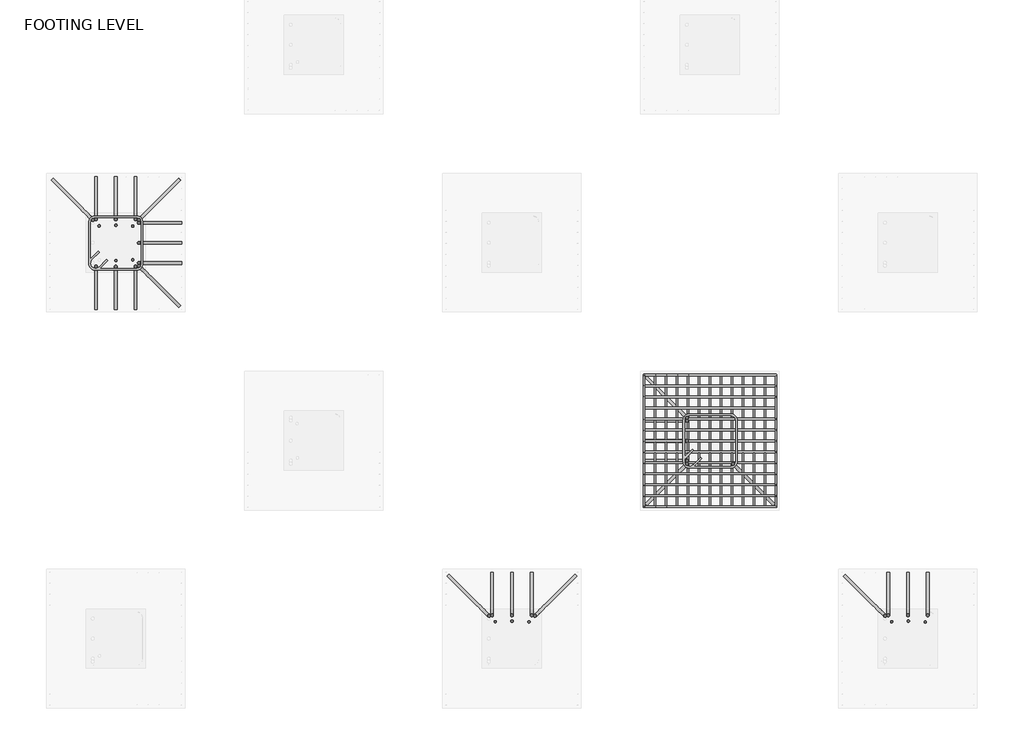
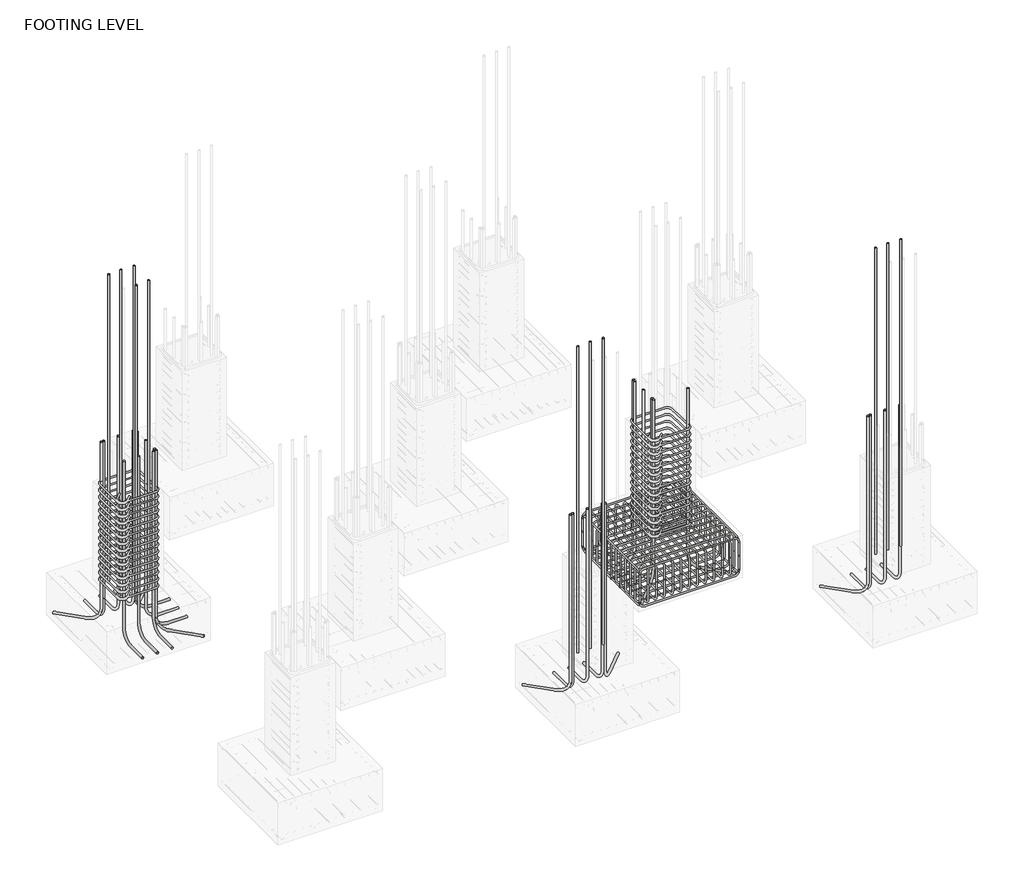
# One storey, part 5 of 10: 33 reinforcing bars.
"""IFC4 building model written with IfcOpenShell, lengths in millimetres."""

from ifc_helpers import new_model, si_unit, point, frame, origin, place, context, project, spatial, polyline, circle_curve, trimmed, segment, composite_curve, source, transform, mapped, element, save
from ifc_brep_helpers import swept_disk

model = new_model("IFC4")

# Units and contexts
model_context = context("Model", 3, world=origin())
ifc_project = project(units=[si_unit("LENGTHUNIT", "METRE", prefix="MILLI")], contexts=[model_context])

# Site, building, storey
site = spatial("IfcSite", under=ifc_project)
building = spatial("IfcBuilding", under=site)
storey = spatial("IfcBuildingStorey", under=building, Name="FOOTING LEVEL", Elevation=-2133.6)

# Reinforcing bars
placement = place(None, origin())
reinforcing_bar_shape = source(origin(), model_context, "Body", "SolidModel", [
    swept_disk(composite_curve([segment(polyline([(-2682.9269037, 3804.4829396, -2583.0), (-2682.9269037, 3804.4829396, -2905.1)]), True, "CONTINUOUS"), segment(trimmed(circle_curve(frame((-2773.1269037, 3804.4829396, -2905.1), z_axis=(0.0, 1.0, 0.0), x_axis=(90.20000000000027, 0.0, 0.0)), 90.2), [point((-2682.9269037, 3804.4829396, -2905.1))], [point((-2773.1269037, 3804.4829396, -2995.3))], True, "CARTESIAN"), True, "CONTINUOUS"), segment(polyline([(-2773.1269037, 3804.4829396, -2995.3), (-4620.9269037, 3804.4829396, -2995.3)]), True, "CONTINUOUS"), segment(trimmed(circle_curve(frame((-4620.9269037, 3804.4829396, -2905.1), z_axis=(0.0, 1.0, 0.0), x_axis=(0.0, 0.0, -90.20000000000027)), 90.2), [point((-4620.9269037, 3804.4829396, -2995.3))], [point((-4711.1269037, 3804.4829396, -2905.1))], True, "CARTESIAN"), True, "CONTINUOUS"), segment(polyline([(-4711.1269037, 3804.4829396, -2905.1), (-4711.1269037, 3804.4829396, -2583.0)]), True, "CONTINUOUS")], self_intersect=False), 12.7),
])
element("IfcReinforcingBar", 1, at=placement, inside=storey, context=model_context, shape_type="MappedRepresentation", body=[
    mapped(reinforcing_bar_shape, transform((0.0, 0.0, 0.0), x_axis=(1.0, 0.0, 0.0), y_axis=(0.0, 1.0, 0.0), z_axis=(0.0, 0.0, 1.0))),
    mapped(reinforcing_bar_shape, transform((0.0, -169.0166667, 0.0), x_axis=(1.0, 0.0, 0.0), y_axis=(0.0, 1.0, 0.0), z_axis=(0.0, 0.0, 1.0))),
    mapped(reinforcing_bar_shape, transform((0.0, -338.0333333, 0.0), x_axis=(1.0, 0.0, 0.0), y_axis=(0.0, 1.0, 0.0), z_axis=(0.0, 0.0, 1.0))),
    mapped(reinforcing_bar_shape, transform((0.0, -507.05, 0.0), x_axis=(1.0, 0.0, 0.0), y_axis=(0.0, 1.0, 0.0), z_axis=(0.0, 0.0, 1.0))),
    mapped(reinforcing_bar_shape, transform((0.0, -676.0666667, 0.0), x_axis=(1.0, 0.0, 0.0), y_axis=(0.0, 1.0, 0.0), z_axis=(0.0, 0.0, 1.0))),
    mapped(reinforcing_bar_shape, transform((0.0, -845.0833333, 0.0), x_axis=(1.0, 0.0, 0.0), y_axis=(0.0, 1.0, 0.0), z_axis=(0.0, 0.0, 1.0))),
    mapped(reinforcing_bar_shape, transform((0.0, -1014.1, 0.0), x_axis=(1.0, 0.0, 0.0), y_axis=(0.0, 1.0, 0.0), z_axis=(0.0, 0.0, 1.0))),
    mapped(reinforcing_bar_shape, transform((0.0, -1183.1166667, 0.0), x_axis=(1.0, 0.0, 0.0), y_axis=(0.0, 1.0, 0.0), z_axis=(0.0, 0.0, 1.0))),
    mapped(reinforcing_bar_shape, transform((0.0, -1352.1333333, 0.0), x_axis=(1.0, 0.0, 0.0), y_axis=(0.0, 1.0, 0.0), z_axis=(0.0, 0.0, 1.0))),
    mapped(reinforcing_bar_shape, transform((0.0, -1521.15, 0.0), x_axis=(1.0, 0.0, 0.0), y_axis=(0.0, 1.0, 0.0), z_axis=(0.0, 0.0, 1.0))),
    mapped(reinforcing_bar_shape, transform((0.0, -1690.1666667, 0.0), x_axis=(1.0, 0.0, 0.0), y_axis=(0.0, 1.0, 0.0), z_axis=(0.0, 0.0, 1.0))),
    mapped(reinforcing_bar_shape, transform((0.0, -1859.1833333, 0.0), x_axis=(1.0, 0.0, 0.0), y_axis=(0.0, 1.0, 0.0), z_axis=(0.0, 0.0, 1.0))),
    mapped(reinforcing_bar_shape, transform((0.0, -2028.2, 0.0), x_axis=(1.0, 0.0, 0.0), y_axis=(0.0, 1.0, 0.0), z_axis=(0.0, 0.0, 1.0))),
])
reinforcing_bar_2_shape = source(origin(), model_context, "Body", "SolidModel", [
    swept_disk(composite_curve([segment(polyline([(-4711.1269037, 3804.4829396, -2598.6), (-4711.1269037, 3804.4829396, -2276.5)]), True, "CONTINUOUS"), segment(trimmed(circle_curve(frame((-4620.9269037, 3804.4829396, -2276.5), z_axis=(0.0, 1.0, 0.0), x_axis=(-90.19999999999982, 0.0, 0.0)), 90.2), [point((-4711.1269037, 3804.4829396, -2276.5))], [point((-4620.9269037, 3804.4829396, -2186.3))], True, "CARTESIAN"), True, "CONTINUOUS"), segment(polyline([(-4620.9269037, 3804.4829396, -2186.3), (-2773.1269037, 3804.4829396, -2186.3)]), True, "CONTINUOUS"), segment(trimmed(circle_curve(frame((-2773.1269037, 3804.4829396, -2276.5), z_axis=(0.0, 1.0, 0.0), x_axis=(0.0, 0.0, 90.19999999999982)), 90.2), [point((-2773.1269037, 3804.4829396, -2186.3))], [point((-2682.9269037, 3804.4829396, -2276.5))], True, "CARTESIAN"), True, "CONTINUOUS"), segment(polyline([(-2682.9269037, 3804.4829396, -2276.5), (-2682.9269037, 3804.4829396, -2598.6)]), True, "CONTINUOUS")], self_intersect=False), 12.7),
])
element("IfcReinforcingBar", 2, at=placement, inside=storey, context=model_context, shape_type="MappedRepresentation", body=[
    mapped(reinforcing_bar_2_shape, transform((0.0, 0.0, 0.0), x_axis=(1.0, 0.0, 0.0), y_axis=(0.0, 1.0, 0.0), z_axis=(0.0, 0.0, 1.0))),
    mapped(reinforcing_bar_2_shape, transform((0.0, -169.0166667, 0.0), x_axis=(1.0, 0.0, 0.0), y_axis=(0.0, 1.0, 0.0), z_axis=(0.0, 0.0, 1.0))),
    mapped(reinforcing_bar_2_shape, transform((0.0, -338.0333333, 0.0), x_axis=(1.0, 0.0, 0.0), y_axis=(0.0, 1.0, 0.0), z_axis=(0.0, 0.0, 1.0))),
    mapped(reinforcing_bar_2_shape, transform((0.0, -507.05, 0.0), x_axis=(1.0, 0.0, 0.0), y_axis=(0.0, 1.0, 0.0), z_axis=(0.0, 0.0, 1.0))),
    mapped(reinforcing_bar_2_shape, transform((0.0, -676.0666667, 0.0), x_axis=(1.0, 0.0, 0.0), y_axis=(0.0, 1.0, 0.0), z_axis=(0.0, 0.0, 1.0))),
    mapped(reinforcing_bar_2_shape, transform((0.0, -845.0833333, 0.0), x_axis=(1.0, 0.0, 0.0), y_axis=(0.0, 1.0, 0.0), z_axis=(0.0, 0.0, 1.0))),
    mapped(reinforcing_bar_2_shape, transform((0.0, -1014.1, 0.0), x_axis=(1.0, 0.0, 0.0), y_axis=(0.0, 1.0, 0.0), z_axis=(0.0, 0.0, 1.0))),
    mapped(reinforcing_bar_2_shape, transform((0.0, -1183.1166667, 0.0), x_axis=(1.0, 0.0, 0.0), y_axis=(0.0, 1.0, 0.0), z_axis=(0.0, 0.0, 1.0))),
    mapped(reinforcing_bar_2_shape, transform((0.0, -1352.1333333, 0.0), x_axis=(1.0, 0.0, 0.0), y_axis=(0.0, 1.0, 0.0), z_axis=(0.0, 0.0, 1.0))),
    mapped(reinforcing_bar_2_shape, transform((0.0, -1521.15, 0.0), x_axis=(1.0, 0.0, 0.0), y_axis=(0.0, 1.0, 0.0), z_axis=(0.0, 0.0, 1.0))),
    mapped(reinforcing_bar_2_shape, transform((0.0, -1690.1666667, 0.0), x_axis=(1.0, 0.0, 0.0), y_axis=(0.0, 1.0, 0.0), z_axis=(0.0, 0.0, 1.0))),
    mapped(reinforcing_bar_2_shape, transform((0.0, -1859.1833333, 0.0), x_axis=(1.0, 0.0, 0.0), y_axis=(0.0, 1.0, 0.0), z_axis=(0.0, 0.0, 1.0))),
    mapped(reinforcing_bar_2_shape, transform((0.0, -2028.2, 0.0), x_axis=(1.0, 0.0, 0.0), y_axis=(0.0, 1.0, 0.0), z_axis=(0.0, 0.0, 1.0))),
])
reinforcing_bar_3_shape = source(origin(), model_context, "Body", "SolidModel", [
    swept_disk(composite_curve([segment(polyline([(-2682.9269037, 1776.2829396, -2559.4978077), (-2682.9269037, 1776.2829396, -2881.5978077)]), True, "CONTINUOUS"), segment(trimmed(circle_curve(frame((-2682.9269037, 1866.4829396, -2881.5978077), z_axis=(1.0, 0.0, 0.0), x_axis=(0.0, -90.20000000000005, 0.0)), 90.2), [point((-2682.9269037, 1776.2829396, -2881.5978077))], [point((-2682.9269037, 1866.4829396, -2971.7978077))], True, "CARTESIAN"), True, "CONTINUOUS"), segment(polyline([(-2682.9269037, 1866.4829396, -2971.7978077), (-2682.9269037, 3714.2829396, -2971.7978077)]), True, "CONTINUOUS"), segment(trimmed(circle_curve(frame((-2682.9269037, 3714.2829396, -2881.5978077), z_axis=(1.0, 0.0, 0.0), x_axis=(0.0, 0.0, -90.19999999999982)), 90.2), [point((-2682.9269037, 3714.2829396, -2971.7978077))], [point((-2682.9269037, 3804.4829396, -2881.5978077))], True, "CARTESIAN"), True, "CONTINUOUS"), segment(polyline([(-2682.9269037, 3804.4829396, -2881.5978077), (-2682.9269037, 3804.4829396, -2559.4978077)]), True, "CONTINUOUS")], self_intersect=False), 12.7),
])
element("IfcReinforcingBar", 3, at=placement, inside=storey, context=model_context, shape_type="MappedRepresentation", body=[
    mapped(reinforcing_bar_3_shape, transform((0.0, 0.0, 0.0), x_axis=(1.0, 0.0, 0.0), y_axis=(0.0, 1.0, 0.0), z_axis=(0.0, 0.0, 1.0))),
    mapped(reinforcing_bar_3_shape, transform((-169.0166667, 0.0, 0.0), x_axis=(1.0, 0.0, 0.0), y_axis=(0.0, 1.0, 0.0), z_axis=(0.0, 0.0, 1.0))),
    mapped(reinforcing_bar_3_shape, transform((-338.0333333, 0.0, 0.0), x_axis=(1.0, 0.0, 0.0), y_axis=(0.0, 1.0, 0.0), z_axis=(0.0, 0.0, 1.0))),
    mapped(reinforcing_bar_3_shape, transform((-507.05, 0.0, 0.0), x_axis=(1.0, 0.0, 0.0), y_axis=(0.0, 1.0, 0.0), z_axis=(0.0, 0.0, 1.0))),
    mapped(reinforcing_bar_3_shape, transform((-676.0666667, 0.0, 0.0), x_axis=(1.0, 0.0, 0.0), y_axis=(0.0, 1.0, 0.0), z_axis=(0.0, 0.0, 1.0))),
    mapped(reinforcing_bar_3_shape, transform((-845.0833333, 0.0, 0.0), x_axis=(1.0, 0.0, 0.0), y_axis=(0.0, 1.0, 0.0), z_axis=(0.0, 0.0, 1.0))),
    mapped(reinforcing_bar_3_shape, transform((-1014.1, 0.0, 0.0), x_axis=(1.0, 0.0, 0.0), y_axis=(0.0, 1.0, 0.0), z_axis=(0.0, 0.0, 1.0))),
    mapped(reinforcing_bar_3_shape, transform((-1183.1166667, 0.0, 0.0), x_axis=(1.0, 0.0, 0.0), y_axis=(0.0, 1.0, 0.0), z_axis=(0.0, 0.0, 1.0))),
    mapped(reinforcing_bar_3_shape, transform((-1352.1333333, 0.0, 0.0), x_axis=(1.0, 0.0, 0.0), y_axis=(0.0, 1.0, 0.0), z_axis=(0.0, 0.0, 1.0))),
    mapped(reinforcing_bar_3_shape, transform((-1521.15, 0.0, 0.0), x_axis=(1.0, 0.0, 0.0), y_axis=(0.0, 1.0, 0.0), z_axis=(0.0, 0.0, 1.0))),
    mapped(reinforcing_bar_3_shape, transform((-1690.1666667, 0.0, 0.0), x_axis=(1.0, 0.0, 0.0), y_axis=(0.0, 1.0, 0.0), z_axis=(0.0, 0.0, 1.0))),
    mapped(reinforcing_bar_3_shape, transform((-1859.1833333, 0.0, 0.0), x_axis=(1.0, 0.0, 0.0), y_axis=(0.0, 1.0, 0.0), z_axis=(0.0, 0.0, 1.0))),
    mapped(reinforcing_bar_3_shape, transform((-2028.2, 0.0, 0.0), x_axis=(1.0, 0.0, 0.0), y_axis=(0.0, 1.0, 0.0), z_axis=(0.0, 0.0, 1.0))),
])
reinforcing_bar_4_shape = source(origin(), model_context, "Body", "SolidModel", [
    swept_disk(composite_curve([segment(polyline([(-4711.1269037, 1776.2829396, -2622.9919875), (-4711.1269037, 1776.2829396, -2300.8919875)]), True, "CONTINUOUS"), segment(trimmed(circle_curve(frame((-4711.1269037, 1866.4829396, -2300.8919875), z_axis=(-1.0, 0.0, 0.0), x_axis=(0.0, -90.20000000000005, 0.0)), 90.2), [point((-4711.1269037, 1776.2829396, -2300.8919875))], [point((-4711.1269037, 1866.4829396, -2210.6919875))], True, "CARTESIAN"), True, "CONTINUOUS"), segment(polyline([(-4711.1269037, 1866.4829396, -2210.6919875), (-4711.1269037, 3714.2829396, -2210.6919875)]), True, "CONTINUOUS"), segment(trimmed(circle_curve(frame((-4711.1269037, 3714.2829396, -2300.8919875), z_axis=(-1.0, 0.0, 0.0), x_axis=(0.0, 0.0, 90.20000000000027)), 90.2), [point((-4711.1269037, 3714.2829396, -2210.6919875))], [point((-4711.1269037, 3804.4829396, -2300.8919875))], True, "CARTESIAN"), True, "CONTINUOUS"), segment(polyline([(-4711.1269037, 3804.4829396, -2300.8919875), (-4711.1269037, 3804.4829396, -2622.9919875)]), True, "CONTINUOUS")], self_intersect=False), 12.7),
])
element("IfcReinforcingBar", 4, at=placement, inside=storey, context=model_context, shape_type="MappedRepresentation", body=[
    mapped(reinforcing_bar_4_shape, transform((0.0, 0.0, 0.0), x_axis=(1.0, 0.0, 0.0), y_axis=(0.0, 1.0, 0.0), z_axis=(0.0, 0.0, 1.0))),
    mapped(reinforcing_bar_4_shape, transform((169.0166667, 0.0, 0.0), x_axis=(1.0, 0.0, 0.0), y_axis=(0.0, 1.0, 0.0), z_axis=(0.0, 0.0, 1.0))),
    mapped(reinforcing_bar_4_shape, transform((338.0333333, 0.0, 0.0), x_axis=(1.0, 0.0, 0.0), y_axis=(0.0, 1.0, 0.0), z_axis=(0.0, 0.0, 1.0))),
    mapped(reinforcing_bar_4_shape, transform((507.05, 0.0, 0.0), x_axis=(1.0, 0.0, 0.0), y_axis=(0.0, 1.0, 0.0), z_axis=(0.0, 0.0, 1.0))),
    mapped(reinforcing_bar_4_shape, transform((676.0666667, 0.0, 0.0), x_axis=(1.0, 0.0, 0.0), y_axis=(0.0, 1.0, 0.0), z_axis=(0.0, 0.0, 1.0))),
    mapped(reinforcing_bar_4_shape, transform((845.0833333, 0.0, 0.0), x_axis=(1.0, 0.0, 0.0), y_axis=(0.0, 1.0, 0.0), z_axis=(0.0, 0.0, 1.0))),
    mapped(reinforcing_bar_4_shape, transform((1014.1, 0.0, 0.0), x_axis=(1.0, 0.0, 0.0), y_axis=(0.0, 1.0, 0.0), z_axis=(0.0, 0.0, 1.0))),
    mapped(reinforcing_bar_4_shape, transform((1183.1166667, 0.0, 0.0), x_axis=(1.0, 0.0, 0.0), y_axis=(0.0, 1.0, 0.0), z_axis=(0.0, 0.0, 1.0))),
    mapped(reinforcing_bar_4_shape, transform((1352.1333333, 0.0, 0.0), x_axis=(1.0, 0.0, 0.0), y_axis=(0.0, 1.0, 0.0), z_axis=(0.0, 0.0, 1.0))),
    mapped(reinforcing_bar_4_shape, transform((1521.15, 0.0, 0.0), x_axis=(1.0, 0.0, 0.0), y_axis=(0.0, 1.0, 0.0), z_axis=(0.0, 0.0, 1.0))),
    mapped(reinforcing_bar_4_shape, transform((1690.1666667, 0.0, 0.0), x_axis=(1.0, 0.0, 0.0), y_axis=(0.0, 1.0, 0.0), z_axis=(0.0, 0.0, 1.0))),
    mapped(reinforcing_bar_4_shape, transform((1859.1833333, 0.0, 0.0), x_axis=(1.0, 0.0, 0.0), y_axis=(0.0, 1.0, 0.0), z_axis=(0.0, 0.0, 1.0))),
    mapped(reinforcing_bar_4_shape, transform((2028.2, 0.0, 0.0), x_axis=(1.0, 0.0, 0.0), y_axis=(0.0, 1.0, 0.0), z_axis=(0.0, 0.0, 1.0))),
])
reinforcing_bar_5_shape = source(origin(), model_context, "Body", "SolidModel", [
    swept_disk(composite_curve([segment(polyline([(-12978.1462687, 5573.7015113, 0.0), (-13091.545872, 5460.3019079, 0.0)]), True, "CONTINUOUS"), segment(trimmed(circle_curve(frame((-13155.3269037, 5524.0829396, 0.0), z_axis=(0.0, 0.0, -1.0), x_axis=(63.78103169999849, -63.78103170000031, 0.0)), 90.2), [point((-13091.545872, 5460.3019079, 0.0))], [point((-13245.5269037, 5524.0829396, 0.0))], True, "CARTESIAN"), True, "CONTINUOUS"), segment(polyline([(-13245.5269037, 5524.0829396, 0.0), (-13245.5269037, 6152.6829396, 0.0)]), True, "CONTINUOUS"), segment(trimmed(circle_curve(frame((-13155.3269037, 6152.6829396, 0.0), z_axis=(0.0, 0.0, -1.0), x_axis=(-90.20000000000073, 0.0, 0.0)), 90.2), [point((-13245.5269037, 6152.6829396, 0.0))], [point((-13155.3269037, 6242.8829396, 0.0))], True, "CARTESIAN"), True, "CONTINUOUS"), segment(polyline([(-13155.3269037, 6242.8829396, 0.0), (-12526.7269037, 6242.8829396, 0.0)]), True, "CONTINUOUS"), segment(trimmed(circle_curve(frame((-12526.7269037, 6152.7273645, 2.8305953), z_axis=(0.0, -0.03138132276777647, -0.9995074850051623), x_axis=(0.0, 90.15557510000053, -2.8305953)), 90.2), [point((-12526.7269037, 6242.8829396, 0.0))], [point((-12436.5269037, 6152.7273645, 2.8305953))], True, "CARTESIAN"), True, "CONTINUOUS"), segment(polyline([(-12436.5269037, 6152.7273645, 2.8305953), (-12436.5269037, 5524.0385147, 22.5694047)]), True, "CONTINUOUS"), segment(trimmed(circle_curve(frame((-12526.7269037, 5524.0385147, 22.5694047), z_axis=(0.0, -0.03138132276777647, -0.9995074850051623), x_axis=(90.20000000000073, 0.0, 0.0)), 90.2), [point((-12436.5269037, 5524.0385147, 22.5694047))], [point((-12526.7269037, 5433.8829396, 25.4))], True, "CARTESIAN"), True, "CONTINUOUS"), segment(polyline([(-12526.7269037, 5433.8829396, 25.4), (-13155.3269037, 5433.8829396, 25.4)]), True, "CONTINUOUS"), segment(trimmed(circle_curve(frame((-13155.3269037, 5524.0829396, 25.4), z_axis=(0.0, 0.0, -1.0), x_axis=(0.0, -90.19999999999982, 0.0)), 90.2), [point((-13155.3269037, 5433.8829396, 25.4))], [point((-13219.1079353, 5587.8639713, 25.4))], True, "CARTESIAN"), True, "CONTINUOUS"), segment(polyline([(-13219.1079353, 5587.8639713, 25.4), (-13105.708332, 5701.2635746, 25.4)]), True, "CONTINUOUS")], self_intersect=False), 12.7),
])
element("IfcReinforcingBar", 5, at=placement, inside=storey, context=model_context, shape_type="MappedRepresentation", body=[
    mapped(reinforcing_bar_5_shape, transform((0.0, 0.0, 0.0), x_axis=(1.0, 0.0, 0.0), y_axis=(0.0, 1.0, 0.0), z_axis=(0.0, 0.0, 1.0))),
    mapped(reinforcing_bar_5_shape, transform((0.0, 0.0, -148.6357143), x_axis=(1.0, 0.0, 0.0), y_axis=(0.0, 1.0, 0.0), z_axis=(0.0, 0.0, 1.0))),
    mapped(reinforcing_bar_5_shape, transform((0.0, 0.0, -297.2714286), x_axis=(1.0, 0.0, 0.0), y_axis=(0.0, 1.0, 0.0), z_axis=(0.0, 0.0, 1.0))),
    mapped(reinforcing_bar_5_shape, transform((0.0, 0.0, -445.9071429), x_axis=(1.0, 0.0, 0.0), y_axis=(0.0, 1.0, 0.0), z_axis=(0.0, 0.0, 1.0))),
    mapped(reinforcing_bar_5_shape, transform((0.0, 0.0, -594.5428571), x_axis=(1.0, 0.0, 0.0), y_axis=(0.0, 1.0, 0.0), z_axis=(0.0, 0.0, 1.0))),
    mapped(reinforcing_bar_5_shape, transform((0.0, 0.0, -743.1785714), x_axis=(1.0, 0.0, 0.0), y_axis=(0.0, 1.0, 0.0), z_axis=(0.0, 0.0, 1.0))),
    mapped(reinforcing_bar_5_shape, transform((0.0, 0.0, -891.8142857), x_axis=(1.0, 0.0, 0.0), y_axis=(0.0, 1.0, 0.0), z_axis=(0.0, 0.0, 1.0))),
    mapped(reinforcing_bar_5_shape, transform((0.0, 0.0, -1040.45), x_axis=(1.0, 0.0, 0.0), y_axis=(0.0, 1.0, 0.0), z_axis=(0.0, 0.0, 1.0))),
    mapped(reinforcing_bar_5_shape, transform((0.0, 0.0, -1189.0857143), x_axis=(1.0, 0.0, 0.0), y_axis=(0.0, 1.0, 0.0), z_axis=(0.0, 0.0, 1.0))),
    mapped(reinforcing_bar_5_shape, transform((0.0, 0.0, -1337.7214286), x_axis=(1.0, 0.0, 0.0), y_axis=(0.0, 1.0, 0.0), z_axis=(0.0, 0.0, 1.0))),
    mapped(reinforcing_bar_5_shape, transform((0.0, 0.0, -1486.3571429), x_axis=(1.0, 0.0, 0.0), y_axis=(0.0, 1.0, 0.0), z_axis=(0.0, 0.0, 1.0))),
    mapped(reinforcing_bar_5_shape, transform((0.0, 0.0, -1634.9928571), x_axis=(1.0, 0.0, 0.0), y_axis=(0.0, 1.0, 0.0), z_axis=(0.0, 0.0, 1.0))),
    mapped(reinforcing_bar_5_shape, transform((0.0, 0.0, -1783.6285714), x_axis=(1.0, 0.0, 0.0), y_axis=(0.0, 1.0, 0.0), z_axis=(0.0, 0.0, 1.0))),
    mapped(reinforcing_bar_5_shape, transform((0.0, 0.0, -1932.2642857), x_axis=(1.0, 0.0, 0.0), y_axis=(0.0, 1.0, 0.0), z_axis=(0.0, 0.0, 1.0))),
    mapped(reinforcing_bar_5_shape, transform((0.0, 0.0, -2080.9), x_axis=(1.0, 0.0, 0.0), y_axis=(0.0, 1.0, 0.0), z_axis=(0.0, 0.0, 1.0))),
])
reinforcing_bar_6_shape = source(origin(), model_context, "Body", "SolidModel", [
    swept_disk(composite_curve([segment(polyline([(-3834.1462687, 2525.7015113, 0.0), (-3947.545872, 2412.3019079, 0.0)]), True, "CONTINUOUS"), segment(trimmed(circle_curve(frame((-4011.3269037, 2476.0829396, 0.0), z_axis=(0.0, 0.0, -1.0), x_axis=(63.78103169999986, -63.78103169999986, 0.0)), 90.2), [point((-3947.545872, 2412.3019079, 0.0))], [point((-4101.5269037, 2476.0829396, 0.0))], True, "CARTESIAN"), True, "CONTINUOUS"), segment(polyline([(-4101.5269037, 2476.0829396, 0.0), (-4101.5269037, 3104.6829396, 0.0)]), True, "CONTINUOUS"), segment(trimmed(circle_curve(frame((-4011.3269037, 3104.6829396, 0.0), z_axis=(0.0, 0.0, -1.0), x_axis=(-90.19999999999982, 0.0, 0.0)), 90.2), [point((-4101.5269037, 3104.6829396, 0.0))], [point((-4011.3269037, 3194.8829396, 0.0))], True, "CARTESIAN"), True, "CONTINUOUS"), segment(polyline([(-4011.3269037, 3194.8829396, 0.0), (-3382.7269037, 3194.8829396, 0.0)]), True, "CONTINUOUS"), segment(trimmed(circle_curve(frame((-3382.7269037, 3104.7273645, 2.8305953), z_axis=(0.0, -0.03138132276777647, -0.9995074850051623), x_axis=(0.0, 90.15557510000008, -2.8305953)), 90.2), [point((-3382.7269037, 3194.8829396, 0.0))], [point((-3292.5269037, 3104.7273645, 2.8305953))], True, "CARTESIAN"), True, "CONTINUOUS"), segment(polyline([(-3292.5269037, 3104.7273645, 2.8305953), (-3292.5269037, 2476.0385147, 22.5694047)]), True, "CONTINUOUS"), segment(trimmed(circle_curve(frame((-3382.7269037, 2476.0385147, 22.5694047), z_axis=(0.0, -0.03138132276777647, -0.9995074850051623), x_axis=(90.20000000000027, 0.0, 0.0)), 90.2), [point((-3292.5269037, 2476.0385147, 22.5694047))], [point((-3382.7269037, 2385.8829396, 25.4))], True, "CARTESIAN"), True, "CONTINUOUS"), segment(polyline([(-3382.7269037, 2385.8829396, 25.4), (-4011.3269037, 2385.8829396, 25.4)]), True, "CONTINUOUS"), segment(trimmed(circle_curve(frame((-4011.3269037, 2476.0829396, 25.4), z_axis=(0.0, 0.0, -1.0), x_axis=(0.0, -90.19999999999982, 0.0)), 90.2), [point((-4011.3269037, 2385.8829396, 25.4))], [point((-4075.1079353, 2539.8639713, 25.4))], True, "CARTESIAN"), True, "CONTINUOUS"), segment(polyline([(-4075.1079353, 2539.8639713, 25.4), (-3961.708332, 2653.2635746, 25.4)]), True, "CONTINUOUS")], self_intersect=False), 12.7),
])
element("IfcReinforcingBar", 6, at=placement, inside=storey, context=model_context, shape_type="MappedRepresentation", body=[
    mapped(reinforcing_bar_6_shape, transform((0.0, 0.0, 0.0), x_axis=(1.0, 0.0, 0.0), y_axis=(0.0, 1.0, 0.0), z_axis=(0.0, 0.0, 1.0))),
    mapped(reinforcing_bar_6_shape, transform((0.0, 0.0, -148.6357143), x_axis=(1.0, 0.0, 0.0), y_axis=(0.0, 1.0, 0.0), z_axis=(0.0, 0.0, 1.0))),
    mapped(reinforcing_bar_6_shape, transform((0.0, 0.0, -297.2714286), x_axis=(1.0, 0.0, 0.0), y_axis=(0.0, 1.0, 0.0), z_axis=(0.0, 0.0, 1.0))),
    mapped(reinforcing_bar_6_shape, transform((0.0, 0.0, -445.9071429), x_axis=(1.0, 0.0, 0.0), y_axis=(0.0, 1.0, 0.0), z_axis=(0.0, 0.0, 1.0))),
    mapped(reinforcing_bar_6_shape, transform((0.0, 0.0, -594.5428571), x_axis=(1.0, 0.0, 0.0), y_axis=(0.0, 1.0, 0.0), z_axis=(0.0, 0.0, 1.0))),
    mapped(reinforcing_bar_6_shape, transform((0.0, 0.0, -743.1785714), x_axis=(1.0, 0.0, 0.0), y_axis=(0.0, 1.0, 0.0), z_axis=(0.0, 0.0, 1.0))),
    mapped(reinforcing_bar_6_shape, transform((0.0, 0.0, -891.8142857), x_axis=(1.0, 0.0, 0.0), y_axis=(0.0, 1.0, 0.0), z_axis=(0.0, 0.0, 1.0))),
    mapped(reinforcing_bar_6_shape, transform((0.0, 0.0, -1040.45), x_axis=(1.0, 0.0, 0.0), y_axis=(0.0, 1.0, 0.0), z_axis=(0.0, 0.0, 1.0))),
    mapped(reinforcing_bar_6_shape, transform((0.0, 0.0, -1189.0857143), x_axis=(1.0, 0.0, 0.0), y_axis=(0.0, 1.0, 0.0), z_axis=(0.0, 0.0, 1.0))),
    mapped(reinforcing_bar_6_shape, transform((0.0, 0.0, -1337.7214286), x_axis=(1.0, 0.0, 0.0), y_axis=(0.0, 1.0, 0.0), z_axis=(0.0, 0.0, 1.0))),
    mapped(reinforcing_bar_6_shape, transform((0.0, 0.0, -1486.3571429), x_axis=(1.0, 0.0, 0.0), y_axis=(0.0, 1.0, 0.0), z_axis=(0.0, 0.0, 1.0))),
    mapped(reinforcing_bar_6_shape, transform((0.0, 0.0, -1634.9928571), x_axis=(1.0, 0.0, 0.0), y_axis=(0.0, 1.0, 0.0), z_axis=(0.0, 0.0, 1.0))),
    mapped(reinforcing_bar_6_shape, transform((0.0, 0.0, -1783.6285714), x_axis=(1.0, 0.0, 0.0), y_axis=(0.0, 1.0, 0.0), z_axis=(0.0, 0.0, 1.0))),
    mapped(reinforcing_bar_6_shape, transform((0.0, 0.0, -1932.2642857), x_axis=(1.0, 0.0, 0.0), y_axis=(0.0, 1.0, 0.0), z_axis=(0.0, 0.0, 1.0))),
    mapped(reinforcing_bar_6_shape, transform((0.0, 0.0, -2080.9), x_axis=(1.0, 0.0, 0.0), y_axis=(0.0, 1.0, 0.0), z_axis=(0.0, 0.0, 1.0))),
])
element("IfcReinforcingBar", 7, at=placement, inside=storey, context=model_context, shape_type="SolidModel", body=[
    swept_disk(composite_curve([segment(polyline([(-2716.5730107, 1809.9290467, -2976.5), (-3163.5238015, 2256.8798374, -2976.5)]), True, "CONTINUOUS"), segment(trimmed(circle_curve(frame((-3163.5238015, 2256.8798374, -2722.5), z_axis=(0.7071067811865508, 0.7071067811865444, 0.0), x_axis=(0.0, 0.0, -254.0)), 254.0), [point((-3163.5238015, 2256.8798374, -2976.5))], [point((-3343.1289239, 2436.4849599, -2722.5))], True, "CARTESIAN"), True, "CONTINUOUS"), segment(polyline([(-3343.1289239, 2436.4849599, -2722.5), (-3343.1289239, 2436.4849599, 874.4)]), True, "CONTINUOUS")], self_intersect=False), 21.5),
])
element("IfcReinforcingBar", 8, at=placement, inside=storey, context=model_context, shape_type="SolidModel", body=[
    swept_disk(composite_curve([segment(polyline([(-4677.4807966, 1809.9290467, -2976.5), (-4230.5300058, 2256.8798374, -2976.5)]), True, "CONTINUOUS"), segment(trimmed(circle_curve(frame((-4230.5300058, 2256.8798374, -2722.5), z_axis=(0.7071067811865475, -0.7071067811865477, 0.0), x_axis=(0.0, 0.0, -254.0)), 254.0), [point((-4230.5300058, 2256.8798374, -2976.5))], [point((-4050.9248834, 2436.4849599, -2722.5))], True, "CARTESIAN"), True, "CONTINUOUS"), segment(polyline([(-4050.9248834, 2436.4849599, -2722.5), (-4050.9248834, 2436.4849599, 874.4)]), True, "CONTINUOUS")], self_intersect=False), 21.5),
])
element("IfcReinforcingBar", 9, at=placement, inside=storey, context=model_context, shape_type="SolidModel", body=[
    swept_disk(composite_curve([segment(polyline([(-4677.4807966, 3770.8368325, -2976.5), (-4230.5300058, 3323.8860418, -2976.5)]), True, "CONTINUOUS"), segment(trimmed(circle_curve(frame((-4230.5300058, 3323.8860418, -2722.5), z_axis=(-0.7071067811865508, -0.7071067811865444, 0.0), x_axis=(0.0, 0.0, -254.0)), 254.0), [point((-4230.5300058, 3323.8860418, -2976.5))], [point((-4050.9248834, 3144.2809193, -2722.5))], True, "CARTESIAN"), True, "CONTINUOUS"), segment(polyline([(-4050.9248834, 3144.2809193, -2722.5), (-4050.9248834, 3144.2809193, 874.4)]), True, "CONTINUOUS")], self_intersect=False), 21.5),
])
reinforcing_bar_7_shape = source(origin(), model_context, "Body", "SolidModel", [
    swept_disk(composite_curve([segment(polyline([(-4713.8269037, 2482.0019966, -2976.5), (-4304.9248834, 2482.0019966, -2976.5)]), True, "CONTINUOUS"), segment(trimmed(circle_curve(frame((-4304.9248834, 2482.0019966, -2722.5), z_axis=(0.0, -1.0, 0.0), x_axis=(0.0, 0.0, -254.0)), 254.0), [point((-4304.9248834, 2482.0019966, -2976.5))], [point((-4050.9248834, 2482.0019966, -2722.5))], True, "CARTESIAN"), True, "CONTINUOUS"), segment(polyline([(-4050.9248834, 2482.0019966, -2722.5), (-4050.9248834, 2482.0019966, 874.4)]), True, "CONTINUOUS")], self_intersect=False), 21.5),
])
element("IfcReinforcingBar", 10, at=placement, inside=storey, context=model_context, shape_type="MappedRepresentation", body=[
    mapped(reinforcing_bar_7_shape, transform((0.0, 0.0, 0.0), x_axis=(1.0, 0.0, 0.0), y_axis=(0.0, 1.0, 0.0), z_axis=(0.0, 0.0, 1.0))),
    mapped(reinforcing_bar_7_shape, transform((0.0, 309.128507, 0.0), x_axis=(1.0, 0.0, 0.0), y_axis=(0.0, 1.0, 0.0), z_axis=(0.0, 0.0, 1.0))),
    mapped(reinforcing_bar_7_shape, transform((0.0, 618.2570139, 0.0), x_axis=(1.0, 0.0, 0.0), y_axis=(0.0, 1.0, 0.0), z_axis=(0.0, 0.0, 1.0))),
])
element("IfcReinforcingBar", 11, at=placement, inside=storey, context=model_context, shape_type="SolidModel", body=[
    swept_disk(composite_curve([segment(polyline([(-1629.4807966, 722.8368325, -2976.5), (-1182.5300058, 275.8860418, -2976.5)]), True, "CONTINUOUS"), segment(trimmed(circle_curve(frame((-1182.5300058, 275.8860418, -2722.5), z_axis=(-0.7071067811865508, -0.7071067811865444, 0.0), x_axis=(0.0, 0.0, -254.0)), 254.0), [point((-1182.5300058, 275.8860418, -2976.5))], [point((-1002.9248834, 96.2809193, -2722.5))], True, "CARTESIAN"), True, "CONTINUOUS"), segment(polyline([(-1002.9248834, 96.2809193, -2722.5), (-1002.9248834, 96.2809193, 874.4)]), True, "CONTINUOUS")], self_intersect=False), 21.5),
])
reinforcing_bar_8_shape = source(origin(), model_context, "Body", "SolidModel", [
    swept_disk(composite_curve([segment(polyline([(-345.6587573, 767.4257505, -2976.5), (-345.6587573, 358.5237302, -2976.5)]), True, "CONTINUOUS"), segment(trimmed(circle_curve(frame((-345.6587573, 358.5237302, -2722.5), z_axis=(-1.0, 0.0, 0.0), x_axis=(0.0, 0.0, -254.0)), 254.0), [point((-345.6587573, 358.5237302, -2976.5))], [point((-345.6587573, 104.5237302, -2722.5))], True, "CARTESIAN"), True, "CONTINUOUS"), segment(polyline([(-345.6587573, 104.5237302, -2722.5), (-345.6587573, 104.5237302, 874.4)]), True, "CONTINUOUS")], self_intersect=False), 21.5),
])
element("IfcReinforcingBar", 12, at=placement, inside=storey, context=model_context, shape_type="MappedRepresentation", body=[
    mapped(reinforcing_bar_8_shape, transform((0.0, 0.0, 0.0), x_axis=(1.0, 0.0, 0.0), y_axis=(0.0, 1.0, 0.0), z_axis=(0.0, 0.0, 1.0))),
    mapped(reinforcing_bar_8_shape, transform((-304.9765997, 0.0, 0.0), x_axis=(1.0, 0.0, 0.0), y_axis=(0.0, 1.0, 0.0), z_axis=(0.0, 0.0, 1.0))),
    mapped(reinforcing_bar_8_shape, transform((-609.9531995, 0.0, 0.0), x_axis=(1.0, 0.0, 0.0), y_axis=(0.0, 1.0, 0.0), z_axis=(0.0, 0.0, 1.0))),
])
element("IfcReinforcingBar", 13, at=placement, inside=storey, context=model_context, shape_type="SolidModel", body=[
    swept_disk(composite_curve([segment(polyline([(-5764.5730107, 722.8368325, -2976.5), (-6211.5238015, 275.8860418, -2976.5)]), True, "CONTINUOUS"), segment(trimmed(circle_curve(frame((-6211.5238015, 275.8860418, -2722.5), z_axis=(-0.7071067811865475, 0.7071067811865477, 0.0), x_axis=(0.0, 0.0, -254.0)), 254.0), [point((-6211.5238015, 275.8860418, -2976.5))], [point((-6391.1289239, 96.2809193, -2722.5))], True, "CARTESIAN"), True, "CONTINUOUS"), segment(polyline([(-6391.1289239, 96.2809193, -2722.5), (-6391.1289239, 96.2809193, 874.4)]), True, "CONTINUOUS")], self_intersect=False), 21.5),
])
element("IfcReinforcingBar", 14, at=placement, inside=storey, context=model_context, shape_type="SolidModel", body=[
    swept_disk(composite_curve([segment(polyline([(-7725.4807966, 722.8368325, -2976.5), (-7278.5300058, 275.8860418, -2976.5)]), True, "CONTINUOUS"), segment(trimmed(circle_curve(frame((-7278.5300058, 275.8860418, -2722.5), z_axis=(-0.7071067811865508, -0.7071067811865444, 0.0), x_axis=(0.0, 0.0, -254.0)), 254.0), [point((-7278.5300058, 275.8860418, -2976.5))], [point((-7098.9248834, 96.2809193, -2722.5))], True, "CARTESIAN"), True, "CONTINUOUS"), segment(polyline([(-7098.9248834, 96.2809193, -2722.5), (-7098.9248834, 96.2809193, 874.4)]), True, "CONTINUOUS")], self_intersect=False), 21.5),
])
reinforcing_bar_9_shape = source(origin(), model_context, "Body", "SolidModel", [
    swept_disk(composite_curve([segment(polyline([(-6441.6587573, 767.4257505, -2976.5), (-6441.6587573, 358.5237302, -2976.5)]), True, "CONTINUOUS"), segment(trimmed(circle_curve(frame((-6441.6587573, 358.5237302, -2722.5), z_axis=(-1.0, 0.0, 0.0), x_axis=(0.0, 0.0, -254.0)), 254.0), [point((-6441.6587573, 358.5237302, -2976.5))], [point((-6441.6587573, 104.5237302, -2722.5))], True, "CARTESIAN"), True, "CONTINUOUS"), segment(polyline([(-6441.6587573, 104.5237302, -2722.5), (-6441.6587573, 104.5237302, 874.4)]), True, "CONTINUOUS")], self_intersect=False), 21.5),
])
element("IfcReinforcingBar", 15, at=placement, inside=storey, context=model_context, shape_type="MappedRepresentation", body=[
    mapped(reinforcing_bar_9_shape, transform((0.0, 0.0, 0.0), x_axis=(1.0, 0.0, 0.0), y_axis=(0.0, 1.0, 0.0), z_axis=(0.0, 0.0, 1.0))),
    mapped(reinforcing_bar_9_shape, transform((-304.9765997, 0.0, 0.0), x_axis=(1.0, 0.0, 0.0), y_axis=(0.0, 1.0, 0.0), z_axis=(0.0, 0.0, 1.0))),
    mapped(reinforcing_bar_9_shape, transform((-609.9531995, 0.0, 0.0), x_axis=(1.0, 0.0, 0.0), y_axis=(0.0, 1.0, 0.0), z_axis=(0.0, 0.0, 1.0))),
])
element("IfcReinforcingBar", 16, at=placement, inside=storey, context=model_context, shape_type="SolidModel", body=[
    swept_disk(composite_curve([segment(polyline([(-11860.5730107, 4857.9290467, -2976.5), (-12307.5238015, 5304.8798374, -2976.5)]), True, "CONTINUOUS"), segment(trimmed(circle_curve(frame((-12307.5238015, 5304.8798374, -2722.5), z_axis=(0.7071067811865508, 0.7071067811865444, 0.0), x_axis=(0.0, 0.0, -254.0)), 254.0), [point((-12307.5238015, 5304.8798374, -2976.5))], [point((-12487.1289239, 5484.4849599, -2722.5))], True, "CARTESIAN"), True, "CONTINUOUS"), segment(polyline([(-12487.1289239, 5484.4849599, -2722.5), (-12487.1289239, 5484.4849599, 884.4)]), True, "CONTINUOUS")], self_intersect=False), 21.5),
])
element("IfcReinforcingBar", 17, at=placement, inside=storey, context=model_context, shape_type="SolidModel", body=[
    swept_disk(composite_curve([segment(polyline([(-11860.5730107, 6818.8368325, -2976.5), (-12307.5238015, 6371.8860418, -2976.5)]), True, "CONTINUOUS"), segment(trimmed(circle_curve(frame((-12307.5238015, 6371.8860418, -2722.5), z_axis=(-0.7071067811865475, 0.7071067811865477, 0.0), x_axis=(0.0, 0.0, -254.0)), 254.0), [point((-12307.5238015, 6371.8860418, -2976.5))], [point((-12487.1289239, 6192.2809193, -2722.5))], True, "CARTESIAN"), True, "CONTINUOUS"), segment(polyline([(-12487.1289239, 6192.2809193, -2722.5), (-12487.1289239, 6192.2809193, 884.4)]), True, "CONTINUOUS")], self_intersect=False), 21.5),
])
element("IfcReinforcingBar", 18, at=placement, inside=storey, context=model_context, shape_type="SolidModel", body=[
    swept_disk(composite_curve([segment(polyline([(-13821.4807966, 6818.8368325, -2976.5), (-13374.5300058, 6371.8860418, -2976.5)]), True, "CONTINUOUS"), segment(trimmed(circle_curve(frame((-13374.5300058, 6371.8860418, -2722.5), z_axis=(-0.7071067811865508, -0.7071067811865444, 0.0), x_axis=(0.0, 0.0, -254.0)), 254.0), [point((-13374.5300058, 6371.8860418, -2976.5))], [point((-13194.9248834, 6192.2809193, -2722.5))], True, "CARTESIAN"), True, "CONTINUOUS"), segment(polyline([(-13194.9248834, 6192.2809193, -2722.5), (-13194.9248834, 6192.2809193, 884.4)]), True, "CONTINUOUS")], self_intersect=False), 21.5),
])
element("IfcReinforcingBar", 19, at=placement, inside=storey, context=model_context, shape_type="SolidModel", body=[
    swept_disk(composite_curve([segment(polyline([(-11860.5730107, 4857.9290467, -2976.5), (-12307.5238015, 5304.8798374, -2976.5)]), True, "CONTINUOUS"), segment(trimmed(circle_curve(frame((-12307.5238015, 5304.8798374, -2722.5), z_axis=(0.7071067811865508, 0.7071067811865444, 0.0), x_axis=(0.0, 0.0, -254.0)), 254.0), [point((-12307.5238015, 5304.8798374, -2976.5))], [point((-12487.1289239, 5484.4849599, -2722.5))], True, "CARTESIAN"), True, "CONTINUOUS"), segment(polyline([(-12487.1289239, 5484.4849599, -2722.5), (-12487.1289239, 5484.4849599, 884.4)]), True, "CONTINUOUS")], self_intersect=False), 21.5),
])
reinforcing_bar_10_shape = source(origin(), model_context, "Body", "SolidModel", [
    swept_disk(composite_curve([segment(polyline([(-11824.2269037, 5530.0019966, -2976.5), (-12233.1289239, 5530.0019966, -2976.5)]), True, "CONTINUOUS"), segment(trimmed(circle_curve(frame((-12233.1289239, 5530.0019966, -2722.5), z_axis=(0.0, 1.0, 0.0), x_axis=(0.0, 0.0, -254.0)), 254.0), [point((-12233.1289239, 5530.0019966, -2976.5))], [point((-12487.1289239, 5530.0019966, -2722.5))], True, "CARTESIAN"), True, "CONTINUOUS"), segment(polyline([(-12487.1289239, 5530.0019966, -2722.5), (-12487.1289239, 5530.0019966, 884.4)]), True, "CONTINUOUS")], self_intersect=False), 21.5),
])
element("IfcReinforcingBar", 20, at=placement, inside=storey, context=model_context, shape_type="MappedRepresentation", body=[
    mapped(reinforcing_bar_10_shape, transform((0.0, 0.0, 0.0), x_axis=(1.0, 0.0, 0.0), y_axis=(0.0, 1.0, 0.0), z_axis=(0.0, 0.0, 1.0))),
    mapped(reinforcing_bar_10_shape, transform((0.0, 309.128507, 0.0), x_axis=(1.0, 0.0, 0.0), y_axis=(0.0, 1.0, 0.0), z_axis=(0.0, 0.0, 1.0))),
    mapped(reinforcing_bar_10_shape, transform((0.0, 618.2570139, 0.0), x_axis=(1.0, 0.0, 0.0), y_axis=(0.0, 1.0, 0.0), z_axis=(0.0, 0.0, 1.0))),
])
reinforcing_bar_11_shape = source(origin(), model_context, "Body", "SolidModel", [
    swept_disk(composite_curve([segment(polyline([(-12537.6587573, 6863.4257505, -2976.5), (-12537.6587573, 6454.5237302, -2976.5)]), True, "CONTINUOUS"), segment(trimmed(circle_curve(frame((-12537.6587573, 6454.5237302, -2722.5), z_axis=(-1.0, 0.0, 0.0), x_axis=(0.0, 0.0, -254.0)), 254.0), [point((-12537.6587573, 6454.5237302, -2976.5))], [point((-12537.6587573, 6200.5237302, -2722.5))], True, "CARTESIAN"), True, "CONTINUOUS"), segment(polyline([(-12537.6587573, 6200.5237302, -2722.5), (-12537.6587573, 6200.5237302, 884.4)]), True, "CONTINUOUS")], self_intersect=False), 21.5),
])
element("IfcReinforcingBar", 21, at=placement, inside=storey, context=model_context, shape_type="MappedRepresentation", body=[
    mapped(reinforcing_bar_11_shape, transform((0.0, 0.0, 0.0), x_axis=(1.0, 0.0, 0.0), y_axis=(0.0, 1.0, 0.0), z_axis=(0.0, 0.0, 1.0))),
    mapped(reinforcing_bar_11_shape, transform((-304.9765997, 0.0, 0.0), x_axis=(1.0, 0.0, 0.0), y_axis=(0.0, 1.0, 0.0), z_axis=(0.0, 0.0, 1.0))),
    mapped(reinforcing_bar_11_shape, transform((-609.9531995, 0.0, 0.0), x_axis=(1.0, 0.0, 0.0), y_axis=(0.0, 1.0, 0.0), z_axis=(0.0, 0.0, 1.0))),
])
reinforcing_bar_12_shape = source(origin(), model_context, "Body", "SolidModel", [
    swept_disk(composite_curve([segment(polyline([(-12537.6587573, 4813.3401287, -2976.5), (-12537.6587573, 5222.242149, -2976.5)]), True, "CONTINUOUS"), segment(trimmed(circle_curve(frame((-12537.6587573, 5222.242149, -2722.5), z_axis=(1.0, 0.0, 0.0), x_axis=(0.0, 0.0, -254.0)), 254.0), [point((-12537.6587573, 5222.242149, -2976.5))], [point((-12537.6587573, 5476.242149, -2722.5))], True, "CARTESIAN"), True, "CONTINUOUS"), segment(polyline([(-12537.6587573, 5476.242149, -2722.5), (-12537.6587573, 5476.242149, 884.4)]), True, "CONTINUOUS")], self_intersect=False), 21.5),
])
element("IfcReinforcingBar", 22, at=placement, inside=storey, context=model_context, shape_type="MappedRepresentation", body=[
    mapped(reinforcing_bar_12_shape, transform((0.0, 0.0, 0.0), x_axis=(1.0, 0.0, 0.0), y_axis=(0.0, 1.0, 0.0), z_axis=(0.0, 0.0, 1.0))),
    mapped(reinforcing_bar_12_shape, transform((-304.9765997, 0.0, 0.0), x_axis=(1.0, 0.0, 0.0), y_axis=(0.0, 1.0, 0.0), z_axis=(0.0, 0.0, 1.0))),
    mapped(reinforcing_bar_12_shape, transform((-609.9531995, 0.0, 0.0), x_axis=(1.0, 0.0, 0.0), y_axis=(0.0, 1.0, 0.0), z_axis=(0.0, 0.0, 1.0))),
])
element("IfcReinforcingBar", 23, at=placement, inside=storey, context=model_context, shape_type="SolidModel", body=[
    swept_disk(composite_curve([segment(polyline([(-12581.0269037, 6098.3829396, 4538.8488542), (-12581.0269037, 6098.3829396, -2093.6)]), True, "CONTINUOUS")], self_intersect=False), 17.9),
])
element("IfcReinforcingBar", 24, at=placement, inside=storey, context=model_context, shape_type="SolidModel", body=[
    swept_disk(composite_curve([segment(polyline([(-13098.5269037, 6100.8829396, 4538.8488542), (-13098.5269037, 6100.8829396, -2093.6)]), True, "CONTINUOUS")], self_intersect=False), 17.9),
])
element("IfcReinforcingBar", 25, at=placement, inside=storey, context=model_context, shape_type="SolidModel", body=[
    swept_disk(composite_curve([segment(polyline([(-12581.0269037, 5578.3829396, 4538.8488542), (-12581.0269037, 5578.3829396, -2093.6)]), True, "CONTINUOUS")], self_intersect=False), 17.9),
])
element("IfcReinforcingBar", 26, at=placement, inside=storey, context=model_context, shape_type="SolidModel", body=[
    swept_disk(composite_curve([segment(polyline([(-12841.0269037, 6110.8829396, 4538.8488542), (-12841.0269037, 6110.8829396, -2093.6)]), True, "CONTINUOUS")], self_intersect=False), 17.9),
])
element("IfcReinforcingBar", 27, at=placement, inside=storey, context=model_context, shape_type="SolidModel", body=[
    swept_disk(composite_curve([segment(polyline([(-12841.0269037, 5565.8829396, 4538.8488542), (-12841.0269037, 5565.8829396, -2093.6)]), True, "CONTINUOUS")], self_intersect=False), 17.9),
])
element("IfcReinforcingBar", 28, at=placement, inside=storey, context=model_context, shape_type="SolidModel", body=[
    swept_disk(composite_curve([segment(polyline([(-6485.0269037, 2.3829396, 4538.8488542), (-6485.0269037, 2.3829396, -2093.6)]), True, "CONTINUOUS")], self_intersect=False), 17.9),
])
element("IfcReinforcingBar", 29, at=placement, inside=storey, context=model_context, shape_type="SolidModel", body=[
    swept_disk(composite_curve([segment(polyline([(-7002.5269037, 4.8829396, 4538.8488542), (-7002.5269037, 4.8829396, -2093.6)]), True, "CONTINUOUS")], self_intersect=False), 17.9),
])
element("IfcReinforcingBar", 30, at=placement, inside=storey, context=model_context, shape_type="SolidModel", body=[
    swept_disk(composite_curve([segment(polyline([(-6745.0269037, 14.8829396, 4538.8488542), (-6745.0269037, 14.8829396, -2093.6)]), True, "CONTINUOUS")], self_intersect=False), 17.9),
])
element("IfcReinforcingBar", 31, at=placement, inside=storey, context=model_context, shape_type="SolidModel", body=[
    swept_disk(composite_curve([segment(polyline([(-385.0269037, 2.3829396, 4538.8488542), (-385.0269037, 2.3829396, -2093.6)]), True, "CONTINUOUS")], self_intersect=False), 17.9),
])
element("IfcReinforcingBar", 32, at=placement, inside=storey, context=model_context, shape_type="SolidModel", body=[
    swept_disk(composite_curve([segment(polyline([(-902.5269037, 4.8829396, 4538.8488542), (-902.5269037, 4.8829396, -2093.6)]), True, "CONTINUOUS")], self_intersect=False), 17.9),
])
element("IfcReinforcingBar", 33, at=placement, inside=storey, context=model_context, shape_type="SolidModel", body=[
    swept_disk(composite_curve([segment(polyline([(-645.0269037, 14.8829396, 4538.8488542), (-645.0269037, 14.8829396, -2093.6)]), True, "CONTINUOUS")], self_intersect=False), 17.9),
])

save(model, "model.ifc")

# Revit data of these elements
# Elements 1, 2, 3, 4, 5, 6, 7, 8, 9, 10, 11, 12, 13, 14, 15, 16, 17, 18, 19, 20, 21, 22, 23, 24, 25, 26, 27, 28, 29, 30, 31, 32, 33 (IfcReinforcingBar)
#   Phase Created = New Construction
